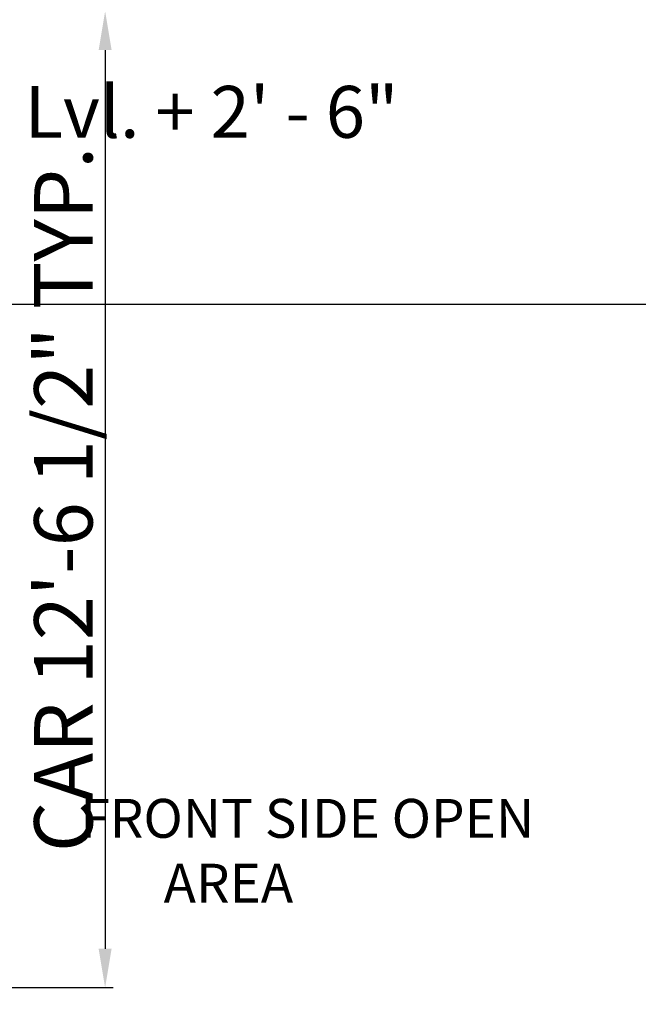
# Model space of a CAD drawing. Units: millimetres. Extents: x 595116 to 630915, y 909473 to 920225.
# Tile 8 of 134: x 629404 to 629500, y 919194 to 919346. Entities that reach past the tile are written whole.
import ezdxf

# ---------------------------------------------------------------- set-up
doc = ezdxf.new("R2010")
doc.units = ezdxf.units.MM
for name, color, linetype, lineweight in [('A-ANNO-SYMB', 7, 'Continuous', 18), ('A-AREA-IDEN', 7, 'Continuous', 20), ('Dimension', 3, 'Continuous', 18)]:
    doc.layers.add(name, color=color, linetype=linetype, lineweight=lineweight)
doc.styles.get("Standard").update_dxf_attribs({"font": 'arial.ttf'})
doc.dimstyles.new('ISO-25', dxfattribs={"dimtxt": 9, "dimasz": 6, "dimexe": 1.25, "dimexo": 0.625, "dimtad": 1, "dimlunit": 4, "dimtxsty": 'Standard', "dimcen": 2.5, "dimadec": 0, "dimazin": 0, "dimtfac": 1, "dimtmove": 0, "dimatfit": 3, "dimfxl": 1, "dimarcsym": 0})

# ---------------------------------------------------------------- blocks, each defined once
blk = doc.blocks.new('*D186')
at = {"layer": 'Defpoints', "color": 0, "transparency": 16777216}
for p in [(629394.93, 919347.24), (629394.93, 919196.66), (629417.52, 919196.66)]:
    blk.add_point(p, dxfattribs=at)
at = {"layer": 'Dimension', "color": 0, "lineweight": -2, "transparency": 16777216}
for p, q in [((629395.55, 919347.24), (629418.77, 919347.24)), ((629417.52, 919341.24), (629417.52, 919202.66)), ((629395.55, 919196.66), (629418.77, 919196.66))]:
    blk.add_line(p, q, dxfattribs=at)
at = {"layer": 'Dimension', "color": 0, "transparency": 16777216}
for points in [[(629416.52, 919341.24), (629418.52, 919341.24), (629417.52, 919347.24)], [(629416.52, 919202.66), (629418.52, 919202.66), (629417.52, 919196.66)]]:
    blk.add_solid(points, dxfattribs=at)
at = {"layer": 'Dimension', "color": 0, "transparency": 16777216, "insert": (629412.24, 919271.95), "char_height": 9, "attachment_point": 5, "rotation": 90}
blk.add_mtext('CAR 12\'-6 1/2" TYP.', dxfattribs=at)
blk = doc.blocks.new('*D215')
at = {"layer": 'Defpoints', "color": 0, "transparency": 16777216}
for p in [(629316.04, 919411.83), (629505.04, 919411.83), (629505.04, 918832.38)]:
    blk.add_point(p, dxfattribs=at)
at = {"layer": 'Dimension', "color": 0, "lineweight": -2, "transparency": 16777216}
for p, q in [((629316.04, 919411.2), (629316.04, 918831.13)), ((629505.04, 919411.2), (629505.04, 918831.13)), ((629322.04, 918832.38), (629499.04, 918832.38))]:
    blk.add_line(p, q, dxfattribs=at)
at = {"layer": 'Dimension', "color": 0, "transparency": 16777216}
for points in [[(629322.04, 918833.38), (629322.04, 918831.38), (629316.04, 918832.38)], [(629499.04, 918833.38), (629499.04, 918831.38), (629505.04, 918832.38)]]:
    blk.add_solid(points, dxfattribs=at)
at = {"layer": 'Dimension', "color": 0, "transparency": 16777216, "insert": (629410.54, 918837.6), "char_height": 9, "attachment_point": 5}
blk.add_mtext('15\'-9"', dxfattribs=at)
blk = doc.blocks.new('*D221')
at = {"layer": 'Defpoints', "color": 0, "transparency": 16777216}
for p in [(629511.27, 919302.01), (629155.38, 919160.92), (629511.27, 919160.92)]:
    blk.add_point(p, dxfattribs=at)
at = {"layer": 'Dimension', "color": 0, "lineweight": -2, "transparency": 16777216}
for p, q in [((629510.65, 919302.01), (629154.13, 919302.01)), ((629155.38, 919296.01), (629155.38, 919166.92)), ((629510.65, 919160.92), (629154.13, 919160.92))]:
    blk.add_line(p, q, dxfattribs=at)
at = {"layer": 'Dimension', "color": 0, "transparency": 16777216}
for points in [[(629154.38, 919296.01), (629156.38, 919296.01), (629155.38, 919302.01)], [(629154.38, 919166.92), (629156.38, 919166.92), (629155.38, 919160.92)]]:
    blk.add_solid(points, dxfattribs=at)
at = {"layer": 'Dimension', "color": 0, "transparency": 16777216, "insert": (629150.16, 919231.46), "char_height": 9, "attachment_point": 5, "rotation": 90}
blk.add_mtext('11\'-9"', dxfattribs=at)

msp = doc.modelspace()

# ---------------------------------------------------------------- texts
at = {"layer": 'A-ANNO-SYMB', "insert": (629390.429, 919335.712), "char_height": 8, "attachment_point": 1}
msp.add_mtext_dynamic_manual_height_columns('{      Lvl. + 2\' - 6"}', width=83.57324, gutter_width=12.5, heights=[0], dxfattribs=at)
at = {"layer": 'A-AREA-IDEN', "insert": (629408.217, 919225.763), "char_height": 6, "attachment_point": 1}
msp.add_mtext_dynamic_manual_height_columns('{   FRONT SIDE OPEN\\P          AREA}', width=83.57324, gutter_width=12.5, heights=[0], dxfattribs=at)

# ---------------------------------------------------------------- dimensions: what is measured, and where the dimension line sits
at = {"layer": 'Dimension'}
dim = msp.add_linear_dim(base=(629505.041, 918832.378), p1=(629316.041, 919411.828), p2=(629505.041, 919411.828), dimstyle='ISO-25', override={"dimdec": 1, "dimlfac": 1, "dimrnd": 0, "dimzin": 1, "dimdsep": 46, "dimlunit": 4, "dimfrac": 2}, dxfattribs=at)
dim.commit()
dim.dimension.update_dxf_attribs({"geometry": '*D215', "text_midpoint": (629410.541, 918837.598)})
dim = msp.add_linear_dim(base=(629417.516, 919196.66), p1=(629394.93, 919347.236), p2=(629394.93, 919196.66), angle=270, text='CAR <> TYP.', dimstyle='ISO-25', override={"dimdec": 1, "dimlfac": 1, "dimrnd": 0, "dimzin": 1, "dimdsep": 46, "dimlunit": 4, "dimfrac": 2}, dxfattribs=at)
dim.commit()
dim.dimension.update_dxf_attribs({"geometry": '*D186', "text_midpoint": (629412.238, 919271.948)})
dim = msp.add_linear_dim(base=(629155.382, 919160.917), p1=(629511.274, 919302.009), p2=(629511.274, 919160.917), angle=90, dimstyle='ISO-25', override={"dimdec": 1, "dimlfac": 1, "dimrnd": 0, "dimzin": 1, "dimdsep": 46, "dimlunit": 4, "dimfrac": 2}, dxfattribs=at)
dim.commit()
dim.dimension.update_dxf_attribs({"geometry": '*D221', "text_midpoint": (629150.162, 919231.463)})

doc.saveas('drawing.dxf')
